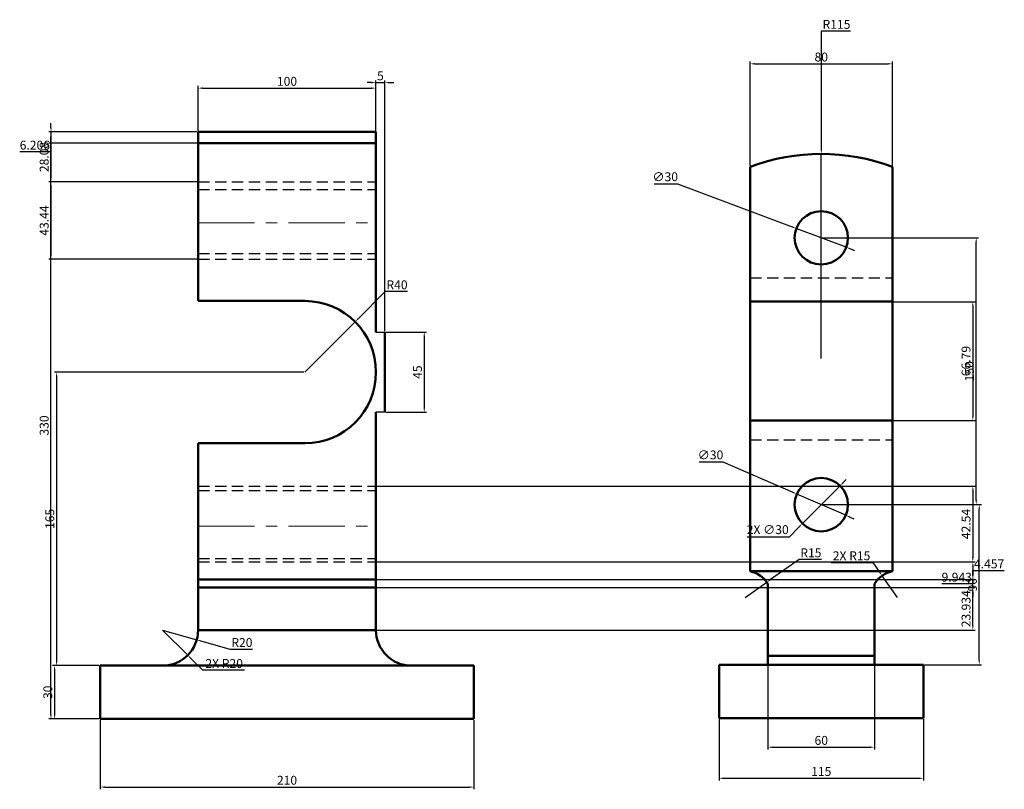
# Model space of a CAD drawing. Units: millimetres. Extents: x 1084 to 2343, y 1141 to 1965.
# Tile 2 of 4: x 1084 to 1638, y 1532 to 1965. Entities that reach past the tile are written whole.
import ezdxf

# ---------------------------------------------------------------- set-up
doc = ezdxf.new("R2010")
doc.units = ezdxf.units.MM
doc.linetypes.add('CENTER', pattern=[50.8, 31.75, -6.35, 6.35, -6.35])
doc.linetypes.add('HIDDEN', pattern=[9.525, 6.35, -3.175])
for name, color, linetype, lineweight in [('M-CNTR', 1, 'CENTER', 18), ('M-DIMS', 2, 'Continuous', 25), ('M-HIDN', 8, 'HIDDEN', 25), ('M-OUTL', 7, 'Continuous', 50)]:
    doc.layers.add(name, color=color, linetype=linetype, lineweight=lineweight)
doc.styles.get("Standard").update_dxf_attribs({"font": 'arial.ttf'})
doc.dimstyles.new('ISO-25', dxfattribs={"dimtxt": 5, "dimasz": 2.5, "dimexe": 1.25, "dimexo": 0.625, "dimtad": 1, "dimtoh": 1, "dimdec": 0, "dimtxsty": 'Standard', "dimcen": 2.5, "dimadec": 0, "dimazin": 0, "dimtfac": 1, "dimtdec": 0, "dimtmove": 0, "dimatfit": 3, "dimfxl": 1, "dimarcsym": 0})

# ---------------------------------------------------------------- blocks, each defined once
blk = doc.blocks.new('*D1')
at = {"layer": 'Defpoints', "color": 0, "transparency": 16777216}
for p in [(1129.73, 1571.53), (1339.73, 1571.53), (1339.73, 1533.25)]:
    blk.add_point(p, dxfattribs=at)
at = {"layer": 'M-DIMS', "color": 0, "lineweight": -2, "transparency": 16777216}
for p, q in [((1129.73, 1570.9), (1129.73, 1532)), ((1339.73, 1570.9), (1339.73, 1532)), ((1132.23, 1533.25), (1337.23, 1533.25))]:
    blk.add_line(p, q, dxfattribs=at)
at = {"layer": 'M-DIMS', "color": 0, "transparency": 16777216}
for points in [[(1132.23, 1533.67), (1132.23, 1532.84), (1129.73, 1533.25)], [(1337.23, 1533.67), (1337.23, 1532.84), (1339.73, 1533.25)]]:
    blk.add_solid(points, dxfattribs=at)
at = {"layer": 'M-DIMS', "color": 0, "transparency": 16777216, "insert": (1234.73, 1536.43), "char_height": 5, "attachment_point": 5}
blk.add_mtext('210', dxfattribs=at)
blk = doc.blocks.new('*D2')
at = {"layer": 'Defpoints', "color": 0, "transparency": 16777216}
for p in [(1129.73, 1601.53), (1104.02, 1571.53), (1129.73, 1571.53)]:
    blk.add_point(p, dxfattribs=at)
at = {"layer": 'M-DIMS', "color": 0, "lineweight": -2, "transparency": 16777216}
for p, q in [((1129.1, 1601.53), (1102.77, 1601.53)), ((1104.02, 1599.03), (1104.02, 1574.03)), ((1129.1, 1571.53), (1102.77, 1571.53))]:
    blk.add_line(p, q, dxfattribs=at)
at = {"layer": 'M-DIMS', "color": 0, "transparency": 16777216}
for points in [[(1103.6, 1599.03), (1104.44, 1599.03), (1104.02, 1601.53)], [(1103.6, 1574.03), (1104.44, 1574.03), (1104.02, 1571.53)]]:
    blk.add_solid(points, dxfattribs=at)
at = {"layer": 'M-DIMS', "color": 0, "transparency": 16777216, "insert": (1100.84, 1586.53), "char_height": 5, "attachment_point": 5, "rotation": 90}
blk.add_mtext('30', dxfattribs=at)
blk = doc.blocks.new('*D3')
at = {"layer": 'Defpoints', "color": 0, "transparency": 16777216}
for p in [(1244.73, 1766.53), (1105.16, 1601.53), (1129.73, 1601.53)]:
    blk.add_point(p, dxfattribs=at)
at = {"layer": 'M-DIMS', "color": 0, "lineweight": -2, "transparency": 16777216}
for p, q in [((1244.1, 1766.53), (1103.91, 1766.53)), ((1105.16, 1764.03), (1105.16, 1604.03)), ((1129.1, 1601.53), (1103.91, 1601.53))]:
    blk.add_line(p, q, dxfattribs=at)
at = {"layer": 'M-DIMS', "color": 0, "transparency": 16777216}
for points in [[(1104.74, 1764.03), (1105.57, 1764.03), (1105.16, 1766.53)], [(1104.74, 1604.03), (1105.57, 1604.03), (1105.16, 1601.53)]]:
    blk.add_solid(points, dxfattribs=at)
at = {"layer": 'M-DIMS', "color": 0, "transparency": 16777216, "insert": (1101.98, 1684.03), "char_height": 5, "attachment_point": 5, "rotation": 90}
blk.add_mtext('165', dxfattribs=at)
blk = doc.blocks.new('*D4')
at = {"layer": 'Defpoints', "color": 0, "transparency": 16777216}
for p in [(1289.73, 1789.03), (1289.73, 1744.03), (1311.91, 1744.03)]:
    blk.add_point(p, dxfattribs=at)
at = {"layer": 'M-DIMS', "color": 0, "lineweight": -2, "transparency": 16777216}
for p, q in [((1290.35, 1789.03), (1313.16, 1789.03)), ((1311.91, 1786.53), (1311.91, 1746.53)), ((1290.35, 1744.03), (1313.16, 1744.03))]:
    blk.add_line(p, q, dxfattribs=at)
at = {"layer": 'M-DIMS', "color": 0, "transparency": 16777216}
for points in [[(1311.49, 1786.53), (1312.32, 1786.53), (1311.91, 1789.03)], [(1311.49, 1746.53), (1312.32, 1746.53), (1311.91, 1744.03)]]:
    blk.add_solid(points, dxfattribs=at)
at = {"layer": 'M-DIMS', "color": 0, "transparency": 16777216, "insert": (1308.74, 1766.53), "char_height": 5, "attachment_point": 5, "rotation": 90}
blk.add_mtext('45', dxfattribs=at)
blk = doc.blocks.new('*D5')
at = {"layer": 'Defpoints', "color": 0, "transparency": 16777216}
for p in [(1284.73, 1926.18), (1184.73, 1901.53), (1284.73, 1901.53)]:
    blk.add_point(p, dxfattribs=at)
at = {"layer": 'M-DIMS', "color": 0, "lineweight": -2, "transparency": 16777216}
for p, q in [((1184.73, 1902.15), (1184.73, 1927.43)), ((1284.73, 1902.15), (1284.73, 1927.43)), ((1187.23, 1926.18), (1282.23, 1926.18))]:
    blk.add_line(p, q, dxfattribs=at)
at = {"layer": 'M-DIMS', "color": 0, "transparency": 16777216}
for points in [[(1187.23, 1926.6), (1187.23, 1925.76), (1184.73, 1926.18)], [(1282.23, 1926.6), (1282.23, 1925.76), (1284.73, 1926.18)]]:
    blk.add_solid(points, dxfattribs=at)
at = {"layer": 'M-DIMS', "color": 0, "transparency": 16777216, "insert": (1234.73, 1929.36), "char_height": 5, "attachment_point": 5}
blk.add_mtext('100', dxfattribs=at)
blk = doc.blocks.new('*D6')
at = {"layer": 'Defpoints', "color": 0, "transparency": 16777216}
for p in [(1164.73, 1621.53), (1183.96, 1616.04)]:
    blk.add_point(p, dxfattribs=at)
at = {"layer": 'M-DIMS', "color": 0, "lineweight": -2, "transparency": 16777216}
for p, q in [((1164.73, 1621.53), (1183.96, 1616.04)), ((1202.75, 1610.68), (1186.36, 1615.35)), ((1215.3, 1610.68), (1202.75, 1610.68))]:
    blk.add_line(p, q, dxfattribs=at)
at = {"layer": 'M-DIMS', "color": 0, "transparency": 16777216}
blk.add_solid([(1186.48, 1615.75), (1186.25, 1614.95), (1183.96, 1616.04)], dxfattribs=at)
at = {"layer": 'M-DIMS', "color": 0, "transparency": 16777216, "insert": (1209.34, 1613.86), "char_height": 5, "attachment_point": 5}
blk.add_mtext('R20', dxfattribs=at)
blk = doc.blocks.new('*D7')
at = {"layer": 'Defpoints', "color": 0, "transparency": 16777216}
for p in [(1477.66, 1572.02), (1592.66, 1572.02), (1592.66, 1538.19)]:
    blk.add_point(p, dxfattribs=at)
at = {"layer": 'M-DIMS', "color": 0, "lineweight": -2, "transparency": 16777216}
for p, q in [((1477.66, 1571.39), (1477.66, 1536.94)), ((1592.66, 1571.39), (1592.66, 1536.94)), ((1480.16, 1538.19), (1590.16, 1538.19))]:
    blk.add_line(p, q, dxfattribs=at)
at = {"layer": 'M-DIMS', "color": 0, "transparency": 16777216}
for points in [[(1480.16, 1538.6), (1480.16, 1537.77), (1477.66, 1538.19)], [(1590.16, 1538.6), (1590.16, 1537.77), (1592.66, 1538.19)]]:
    blk.add_solid(points, dxfattribs=at)
at = {"layer": 'M-DIMS', "color": 0, "transparency": 16777216, "insert": (1535.16, 1541.37), "char_height": 5, "attachment_point": 5}
blk.add_mtext('115', dxfattribs=at)
blk = doc.blocks.new('*D8')
at = {"layer": 'Defpoints', "color": 0, "transparency": 16777216}
for p in [(1505.16, 1602.02), (1565.16, 1602.02), (1565.16, 1555.67)]:
    blk.add_point(p, dxfattribs=at)
at = {"layer": 'M-DIMS', "color": 0, "lineweight": -2, "transparency": 16777216}
for p, q in [((1505.16, 1601.39), (1505.16, 1554.42)), ((1565.16, 1601.39), (1565.16, 1554.42)), ((1507.66, 1555.67), (1562.66, 1555.67))]:
    blk.add_line(p, q, dxfattribs=at)
at = {"layer": 'M-DIMS', "color": 0, "transparency": 16777216}
for points in [[(1507.66, 1556.09), (1507.66, 1555.25), (1505.16, 1555.67)], [(1562.66, 1556.09), (1562.66, 1555.25), (1565.16, 1555.67)]]:
    blk.add_solid(points, dxfattribs=at)
at = {"layer": 'M-DIMS', "color": 0, "transparency": 16777216, "insert": (1535.16, 1558.85), "char_height": 5, "attachment_point": 5}
blk.add_mtext('60', dxfattribs=at)
blk = doc.blocks.new('*D9')
at = {"layer": 'Defpoints', "color": 0, "transparency": 16777216}
for p in [(1535.16, 1692.02), (1624, 1692.02), (1592.66, 1602.02)]:
    blk.add_point(p, dxfattribs=at)
at = {"layer": 'M-DIMS', "color": 0, "lineweight": -2, "transparency": 16777216}
for p, q in [((1535.78, 1692.02), (1625.25, 1692.02)), ((1624, 1604.52), (1624, 1689.52)), ((1593.28, 1602.02), (1625.25, 1602.02))]:
    blk.add_line(p, q, dxfattribs=at)
at = {"layer": 'M-DIMS', "color": 0, "transparency": 16777216}
for points in [[(1623.58, 1689.52), (1624.42, 1689.52), (1624, 1692.02)], [(1623.58, 1604.52), (1624.42, 1604.52), (1624, 1602.02)]]:
    blk.add_solid(points, dxfattribs=at)
at = {"layer": 'M-DIMS', "color": 0, "transparency": 16777216, "insert": (1620.82, 1647.02), "char_height": 5, "attachment_point": 5, "rotation": 90}
blk.add_mtext('90', dxfattribs=at)
blk = doc.blocks.new('*D10')
at = {"layer": 'Defpoints', "color": 0, "transparency": 16777216}
for p in [(1535.16, 1842.02), (1622.3, 1842.02), (1535.16, 1692.02)]:
    blk.add_point(p, dxfattribs=at)
at = {"layer": 'M-DIMS', "color": 0, "lineweight": -2, "transparency": 16777216}
for p, q in [((1535.78, 1842.02), (1623.55, 1842.02)), ((1622.3, 1694.52), (1622.3, 1839.52)), ((1535.78, 1692.02), (1623.55, 1692.02))]:
    blk.add_line(p, q, dxfattribs=at)
at = {"layer": 'M-DIMS', "color": 0, "transparency": 16777216}
for points in [[(1621.89, 1839.52), (1622.72, 1839.52), (1622.3, 1842.02)], [(1621.89, 1694.52), (1622.72, 1694.52), (1622.3, 1692.02)]]:
    blk.add_solid(points, dxfattribs=at)
at = {"layer": 'M-DIMS', "color": 0, "transparency": 16777216, "insert": (1619.12, 1767.02), "char_height": 5, "attachment_point": 5, "rotation": 90}
blk.add_mtext('150', dxfattribs=at)
blk = doc.blocks.new('*D11')
at = {"layer": 'Defpoints', "color": 0, "transparency": 16777216}
for p in [(1575.16, 1939.86), (1495.16, 1882.02), (1575.16, 1882.02)]:
    blk.add_point(p, dxfattribs=at)
at = {"layer": 'M-DIMS', "color": 0, "lineweight": -2, "transparency": 16777216}
for p, q in [((1495.16, 1882.64), (1495.16, 1941.11)), ((1497.66, 1939.86), (1572.66, 1939.86)), ((1575.16, 1882.64), (1575.16, 1941.11))]:
    blk.add_line(p, q, dxfattribs=at)
at = {"layer": 'M-DIMS', "color": 0, "transparency": 16777216}
for points in [[(1497.66, 1940.27), (1497.66, 1939.44), (1495.16, 1939.86)], [(1572.66, 1940.27), (1572.66, 1939.44), (1575.16, 1939.86)]]:
    blk.add_solid(points, dxfattribs=at)
at = {"layer": 'M-DIMS', "color": 0, "transparency": 16777216, "insert": (1535.16, 1943.03), "char_height": 5, "attachment_point": 5}
blk.add_mtext('80', dxfattribs=at)
blk = doc.blocks.new('*D12')
at = {"layer": 'Defpoints', "color": 0, "transparency": 16777216}
for p in [(1521.12, 1847.3), (1549.2, 1836.74)]:
    blk.add_point(p, dxfattribs=at)
at = {"layer": 'M-DIMS', "color": 0, "lineweight": -2, "transparency": 16777216}
for p, q in [((1441.13, 1872.4), (1454.34, 1872.4)), ((1454.34, 1872.4), (1518.78, 1848.18)), ((1549.2, 1836.74), (1521.12, 1847.3)), ((1551.54, 1835.86), (1553.88, 1834.98))]:
    blk.add_line(p, q, dxfattribs=at)
at = {"layer": 'M-DIMS', "color": 0, "transparency": 16777216}
for points in [[(1518.93, 1848.57), (1518.63, 1847.79), (1521.12, 1847.3)], [(1551.69, 1836.25), (1551.39, 1835.47), (1549.2, 1836.74)]]:
    blk.add_solid(points, dxfattribs=at)
at = {"layer": 'M-DIMS', "color": 0, "transparency": 16777216, "insert": (1447.42, 1875.72), "char_height": 5, "attachment_point": 5}
blk.add_mtext('∅30', dxfattribs=at)
blk = doc.blocks.new('*D13')
at = {"layer": 'Defpoints', "color": 0, "transparency": 16777216}
for p in [(1521.4, 1697.99), (1548.92, 1686.05)]:
    blk.add_point(p, dxfattribs=at)
at = {"layer": 'M-DIMS', "color": 0, "lineweight": -2, "transparency": 16777216}
for p, q in [((1466.57, 1716.04), (1479.78, 1716.04)), ((1479.78, 1716.04), (1519.1, 1698.98)), ((1548.92, 1686.05), (1521.4, 1697.99)), ((1551.21, 1685.06), (1553.51, 1684.06))]:
    blk.add_line(p, q, dxfattribs=at)
at = {"layer": 'M-DIMS', "color": 0, "transparency": 16777216}
for points in [[(1519.27, 1699.37), (1518.94, 1698.6), (1521.4, 1697.99)], [(1551.38, 1685.44), (1551.05, 1684.67), (1548.92, 1686.05)]]:
    blk.add_solid(points, dxfattribs=at)
at = {"layer": 'M-DIMS', "color": 0, "transparency": 16777216, "insert": (1472.87, 1719.35), "char_height": 5, "attachment_point": 5}
blk.add_mtext('∅30', dxfattribs=at)
blk = doc.blocks.new('*D14')
at = {"layer": 'Defpoints', "color": 0, "transparency": 16777216}
for p in [(1504.58, 1648.42), (1492.29, 1639.82)]:
    blk.add_point(p, dxfattribs=at)
at = {"layer": 'M-DIMS', "color": 0, "lineweight": -2, "transparency": 16777216}
for p, q in [((1522.72, 1661.12), (1506.63, 1649.86)), ((1535.33, 1661.12), (1522.72, 1661.12)), ((1492.29, 1639.82), (1504.58, 1648.42))]:
    blk.add_line(p, q, dxfattribs=at)
at = {"layer": 'M-DIMS', "color": 0, "transparency": 16777216}
blk.add_solid([(1506.39, 1650.2), (1506.87, 1649.51), (1504.58, 1648.42)], dxfattribs=at)
at = {"layer": 'M-DIMS', "color": 0, "transparency": 16777216, "insert": (1529.34, 1664.3), "char_height": 5, "attachment_point": 5}
blk.add_mtext('R15', dxfattribs=at)
blk = doc.blocks.new('*D48')
at = {"layer": 'Defpoints', "color": 0, "transparency": 16777216}
for p in [(1101.98, 1901.53), (1184.73, 1901.53), (1129.73, 1571.53)]:
    blk.add_point(p, dxfattribs=at)
at = {"layer": 'M-DIMS', "color": 0, "lineweight": -2, "transparency": 16777216}
for p, q in [((1184.1, 1901.53), (1100.73, 1901.53)), ((1101.98, 1574.03), (1101.98, 1899.03)), ((1129.1, 1571.53), (1100.73, 1571.53))]:
    blk.add_line(p, q, dxfattribs=at)
at = {"layer": 'M-DIMS', "color": 0, "transparency": 16777216}
for points in [[(1101.56, 1899.03), (1102.39, 1899.03), (1101.98, 1901.53)], [(1101.56, 1574.03), (1102.39, 1574.03), (1101.98, 1571.53)]]:
    blk.add_solid(points, dxfattribs=at)
at = {"layer": 'M-DIMS', "color": 0, "transparency": 16777216, "insert": (1098.8, 1736.53), "char_height": 5, "attachment_point": 5, "rotation": 90}
blk.add_mtext('330', dxfattribs=at)
blk = doc.blocks.new('*D49')
at = {"layer": 'Defpoints', "color": 0, "transparency": 16777216}
for p in [(1184.73, 1901.53), (1101.98, 1895.32), (1184.73, 1895.32)]:
    blk.add_point(p, dxfattribs=at)
at = {"layer": 'M-DIMS', "color": 0, "lineweight": -2, "transparency": 16777216}
for p, q in [((1101.98, 1904.03), (1101.98, 1906.53)), ((1184.1, 1901.53), (1100.73, 1901.53)), ((1101.98, 1901.53), (1101.98, 1895.32)), ((1184.1, 1895.32), (1100.73, 1895.32)), ((1101.98, 1890.32), (1084.46, 1890.32)), ((1101.98, 1892.82), (1101.98, 1890.32))]:
    blk.add_line(p, q, dxfattribs=at)
at = {"layer": 'M-DIMS', "color": 0, "transparency": 16777216}
for points in [[(1101.56, 1904.03), (1102.39, 1904.03), (1101.98, 1901.53)], [(1101.56, 1892.82), (1102.39, 1892.82), (1101.98, 1895.32)]]:
    blk.add_solid(points, dxfattribs=at)
at = {"layer": 'M-DIMS', "color": 0, "transparency": 16777216, "insert": (1092.9, 1893.5), "char_height": 5, "attachment_point": 5}
blk.add_mtext('6.206', dxfattribs=at)
blk = doc.blocks.new('*D50')
at = {"layer": 'Defpoints', "color": 0, "transparency": 16777216}
for p in [(1289.73, 1929.28), (1284.73, 1789.03), (1289.73, 1789.03)]:
    blk.add_point(p, dxfattribs=at)
at = {"layer": 'M-DIMS', "color": 0, "lineweight": -2, "transparency": 16777216}
for p, q in [((1282.23, 1929.28), (1279.73, 1929.28)), ((1284.73, 1789.65), (1284.73, 1930.53)), ((1284.73, 1929.28), (1289.73, 1929.28)), ((1289.73, 1789.65), (1289.73, 1930.53)), ((1292.23, 1929.28), (1294.73, 1929.28))]:
    blk.add_line(p, q, dxfattribs=at)
at = {"layer": 'M-DIMS', "color": 0, "transparency": 16777216}
for points in [[(1282.23, 1929.69), (1282.23, 1928.86), (1284.73, 1929.28)], [(1292.23, 1929.69), (1292.23, 1928.86), (1289.73, 1929.28)]]:
    blk.add_solid(points, dxfattribs=at)
at = {"layer": 'M-DIMS', "color": 0, "transparency": 16777216, "insert": (1287.23, 1932.45), "char_height": 5, "attachment_point": 5}
blk.add_mtext('5', dxfattribs=at)
blk = doc.blocks.new('*D51')
at = {"layer": 'Defpoints', "color": 0, "transparency": 16777216}
for p in [(1284.73, 1645.46), (1620.41, 1645.46), (1284.73, 1621.53)]:
    blk.add_point(p, dxfattribs=at)
at = {"layer": 'M-DIMS', "color": 0, "lineweight": -2, "transparency": 16777216}
for p, q in [((1285.35, 1645.46), (1621.66, 1645.46)), ((1620.41, 1624.03), (1620.41, 1642.96)), ((1285.35, 1621.53), (1621.66, 1621.53))]:
    blk.add_line(p, q, dxfattribs=at)
at = {"layer": 'M-DIMS', "color": 0, "transparency": 16777216}
for points in [[(1619.99, 1642.96), (1620.83, 1642.96), (1620.41, 1645.46)], [(1619.99, 1624.03), (1620.83, 1624.03), (1620.41, 1621.53)]]:
    blk.add_solid(points, dxfattribs=at)
at = {"layer": 'M-DIMS', "color": 0, "transparency": 16777216, "insert": (1617.23, 1633.5), "char_height": 5, "attachment_point": 5, "rotation": 90}
blk.add_mtext('23.934', dxfattribs=at)
blk = doc.blocks.new('*D52')
at = {"layer": 'Defpoints', "color": 0, "transparency": 16777216}
for p in [(1284.73, 1649.92), (1284.73, 1645.46), (1620.41, 1649.92)]:
    blk.add_point(p, dxfattribs=at)
at = {"layer": 'M-DIMS', "color": 0, "lineweight": -2, "transparency": 16777216}
for p, q in [((1620.41, 1652.42), (1620.41, 1654.92)), ((1620.41, 1654.92), (1638.11, 1654.92)), ((1285.35, 1649.92), (1621.66, 1649.92)), ((1285.35, 1645.46), (1621.66, 1645.46)), ((1620.41, 1645.46), (1620.41, 1649.92)), ((1620.41, 1642.96), (1620.41, 1640.46))]:
    blk.add_line(p, q, dxfattribs=at)
at = {"layer": 'M-DIMS', "color": 0, "transparency": 16777216}
for points in [[(1619.99, 1652.42), (1620.83, 1652.42), (1620.41, 1649.92)], [(1619.99, 1642.96), (1620.83, 1642.96), (1620.41, 1645.46)]]:
    blk.add_solid(points, dxfattribs=at)
at = {"layer": 'M-DIMS', "color": 0, "transparency": 16777216, "insert": (1629.57, 1658.09), "char_height": 5, "attachment_point": 5}
blk.add_mtext('4.457', dxfattribs=at)
blk = doc.blocks.new('*D53')
at = {"layer": 'Defpoints', "color": 0, "transparency": 16777216}
for p in [(1184.73, 1901.53), (1101.98, 1873.45), (1184.73, 1873.45)]:
    blk.add_point(p, dxfattribs=at)
at = {"layer": 'M-DIMS', "color": 0, "lineweight": -2, "transparency": 16777216}
for p, q in [((1184.1, 1901.53), (1100.73, 1901.53)), ((1101.98, 1899.03), (1101.98, 1875.95)), ((1184.1, 1873.45), (1100.73, 1873.45))]:
    blk.add_line(p, q, dxfattribs=at)
at = {"layer": 'M-DIMS', "color": 0, "transparency": 16777216}
for points in [[(1101.56, 1899.03), (1102.39, 1899.03), (1101.98, 1901.53)], [(1101.56, 1875.95), (1102.39, 1875.95), (1101.98, 1873.45)]]:
    blk.add_solid(points, dxfattribs=at)
at = {"layer": 'M-DIMS', "color": 0, "transparency": 16777216, "insert": (1098.8, 1887.49), "char_height": 5, "attachment_point": 5, "rotation": 90}
blk.add_mtext('28.08', dxfattribs=at)
blk = doc.blocks.new('*D54')
at = {"layer": 'Defpoints', "color": 0, "transparency": 16777216}
for p in [(1184.73, 1873.45), (1101.98, 1830.01), (1184.73, 1830.01)]:
    blk.add_point(p, dxfattribs=at)
at = {"layer": 'M-DIMS', "color": 0, "lineweight": -2, "transparency": 16777216}
for p, q in [((1184.1, 1873.45), (1100.73, 1873.45)), ((1101.98, 1870.95), (1101.98, 1832.51)), ((1184.1, 1830.01), (1100.73, 1830.01))]:
    blk.add_line(p, q, dxfattribs=at)
at = {"layer": 'M-DIMS', "color": 0, "transparency": 16777216}
for points in [[(1101.56, 1870.95), (1102.39, 1870.95), (1101.98, 1873.45)], [(1101.56, 1832.51), (1102.39, 1832.51), (1101.98, 1830.01)]]:
    blk.add_solid(points, dxfattribs=at)
at = {"layer": 'M-DIMS', "color": 0, "transparency": 16777216, "insert": (1098.8, 1851.73), "char_height": 5, "attachment_point": 5, "rotation": 90}
blk.add_mtext('43.44', dxfattribs=at)
blk = doc.blocks.new('*D55')
at = {"layer": 'Defpoints', "color": 0, "transparency": 16777216}
for p in [(1284.73, 1702.41), (1284.73, 1659.86), (1620.41, 1659.86)]:
    blk.add_point(p, dxfattribs=at)
at = {"layer": 'M-DIMS', "color": 0, "lineweight": -2, "transparency": 16777216}
for p, q in [((1285.35, 1702.41), (1621.66, 1702.41)), ((1620.41, 1699.91), (1620.41, 1662.36)), ((1285.35, 1659.86), (1621.66, 1659.86))]:
    blk.add_line(p, q, dxfattribs=at)
at = {"layer": 'M-DIMS', "color": 0, "transparency": 16777216}
for points in [[(1619.99, 1699.91), (1620.83, 1699.91), (1620.41, 1702.41)], [(1619.99, 1662.36), (1620.83, 1662.36), (1620.41, 1659.86)]]:
    blk.add_solid(points, dxfattribs=at)
at = {"layer": 'M-DIMS', "color": 0, "transparency": 16777216, "insert": (1617.23, 1681.13), "char_height": 5, "attachment_point": 5, "rotation": 90}
blk.add_mtext('42.54', dxfattribs=at)
blk = doc.blocks.new('*D56')
at = {"layer": 'Defpoints', "color": 0, "transparency": 16777216}
for p in [(1284.73, 1659.86), (1284.73, 1649.92), (1620.41, 1649.92)]:
    blk.add_point(p, dxfattribs=at)
at = {"layer": 'M-DIMS', "color": 0, "lineweight": -2, "transparency": 16777216}
for p, q in [((1285.35, 1659.86), (1621.66, 1659.86)), ((1620.41, 1657.36), (1620.41, 1652.42)), ((1285.35, 1649.92), (1621.66, 1649.92)), ((1620.41, 1647.42), (1602.91, 1647.42)), ((1620.41, 1649.92), (1620.41, 1647.42))]:
    blk.add_line(p, q, dxfattribs=at)
at = {"layer": 'M-DIMS', "color": 0, "transparency": 16777216}
for points in [[(1619.99, 1657.36), (1620.83, 1657.36), (1620.41, 1659.86)], [(1619.99, 1652.42), (1620.83, 1652.42), (1620.41, 1649.92)]]:
    blk.add_solid(points, dxfattribs=at)
at = {"layer": 'M-DIMS', "color": 0, "transparency": 16777216, "insert": (1611.35, 1650.6), "char_height": 5, "attachment_point": 5}
blk.add_mtext('9.943', dxfattribs=at)
blk = doc.blocks.new('*D57')
at = {"layer": 'Defpoints', "color": 0, "transparency": 16777216}
for p in [(1575.16, 1806.14), (1575.16, 1739.35), (1620.41, 1739.35)]:
    blk.add_point(p, dxfattribs=at)
at = {"layer": 'M-DIMS', "color": 0, "lineweight": -2, "transparency": 16777216}
for p, q in [((1575.78, 1806.14), (1621.66, 1806.14)), ((1620.41, 1803.64), (1620.41, 1741.85)), ((1575.78, 1739.35), (1621.66, 1739.35))]:
    blk.add_line(p, q, dxfattribs=at)
at = {"layer": 'M-DIMS', "color": 0, "transparency": 16777216}
for points in [[(1619.99, 1803.64), (1620.83, 1803.64), (1620.41, 1806.14)], [(1619.99, 1741.85), (1620.83, 1741.85), (1620.41, 1739.35)]]:
    blk.add_solid(points, dxfattribs=at)
at = {"layer": 'M-DIMS', "color": 0, "transparency": 16777216, "insert": (1617.23, 1772.75), "char_height": 5, "attachment_point": 5, "rotation": 90}
blk.add_mtext('66.79', dxfattribs=at)
blk = doc.blocks.new('*D69')
at = {"layer": 'Defpoints', "color": 0, "transparency": 16777216}
for p in [(1273.01, 1794.81), (1244.73, 1766.53)]:
    blk.add_point(p, dxfattribs=at)
at = {"layer": 'M-DIMS', "color": 0, "lineweight": -2, "transparency": 16777216}
for p, q in [((1289.98, 1811.78), (1274.78, 1796.58)), ((1302.54, 1811.78), (1289.98, 1811.78)), ((1244.73, 1766.53), (1273.01, 1794.81))]:
    blk.add_line(p, q, dxfattribs=at)
at = {"layer": 'M-DIMS', "color": 0, "transparency": 16777216}
blk.add_solid([(1274.48, 1796.87), (1275.07, 1796.28), (1273.01, 1794.81)], dxfattribs=at)
at = {"layer": 'M-DIMS', "color": 0, "transparency": 16777216, "insert": (1296.57, 1814.96), "char_height": 5, "attachment_point": 5}
blk.add_mtext('R40', dxfattribs=at)
blk = doc.blocks.new('*D70')
at = {"layer": 'Defpoints', "color": 0, "transparency": 16777216}
for p in [(1164.73, 1621.53), (1178.87, 1607.39)]:
    blk.add_point(p, dxfattribs=at)
at = {"layer": 'M-DIMS', "color": 0, "lineweight": -2, "transparency": 16777216}
for p, q in [((1164.73, 1621.53), (1178.87, 1607.39)), ((1187.36, 1598.9), (1180.64, 1605.62)), ((1210.74, 1598.9), (1187.36, 1598.9))]:
    blk.add_line(p, q, dxfattribs=at)
at = {"layer": 'M-DIMS', "color": 0, "transparency": 16777216}
blk.add_solid([(1180.93, 1605.92), (1180.34, 1605.33), (1178.87, 1607.39)], dxfattribs=at)
at = {"layer": 'M-DIMS', "color": 0, "transparency": 16777216, "insert": (1199.36, 1602.08), "char_height": 5, "attachment_point": 5}
blk.add_mtext('2X R20', dxfattribs=at)
blk = doc.blocks.new('*D71')
at = {"layer": 'Defpoints', "color": 0, "transparency": 16777216}
for p in [(1535.16, 1889.2), (1535.16, 1774.2)]:
    blk.add_point(p, dxfattribs=at)
at = {"layer": 'M-DIMS', "color": 0, "lineweight": -2, "transparency": 16777216}
for p, q in [((1551.66, 1958.2), (1535.16, 1958.2)), ((1535.16, 1958.2), (1535.16, 1891.7)), ((1535.16, 1774.2), (1535.16, 1889.2))]:
    blk.add_line(p, q, dxfattribs=at)
at = {"layer": 'M-DIMS', "color": 0, "transparency": 16777216}
blk.add_solid([(1534.74, 1891.7), (1535.58, 1891.7), (1535.16, 1889.2)], dxfattribs=at)
at = {"layer": 'M-DIMS', "color": 0, "transparency": 16777216, "insert": (1543.72, 1961.38), "char_height": 5, "attachment_point": 5}
blk.add_mtext('R115', dxfattribs=at)
blk = doc.blocks.new('*D72')
at = {"layer": 'Defpoints', "color": 0, "transparency": 16777216}
for p in [(1545.74, 1702.66), (1524.58, 1681.38)]:
    blk.add_point(p, dxfattribs=at)
at = {"layer": 'M-DIMS', "color": 0, "lineweight": -2, "transparency": 16777216}
for p, q in [((1547.5, 1704.43), (1549.26, 1706.2)), ((1545.74, 1702.66), (1524.58, 1681.38)), ((1517.26, 1674.02), (1522.82, 1679.61)), ((1493.49, 1674.02), (1517.26, 1674.02))]:
    blk.add_line(p, q, dxfattribs=at)
at = {"layer": 'M-DIMS', "color": 0, "transparency": 16777216}
for points in [[(1547.2, 1704.72), (1547.79, 1704.14), (1545.74, 1702.66)], [(1522.52, 1679.9), (1523.12, 1679.32), (1524.58, 1681.38)]]:
    blk.add_solid(points, dxfattribs=at)
at = {"layer": 'M-DIMS', "color": 0, "transparency": 16777216, "insert": (1505.06, 1677.34), "char_height": 5, "attachment_point": 5}
blk.add_mtext('2X ∅30', dxfattribs=at)
blk = doc.blocks.new('*D73')
at = {"layer": 'Defpoints', "color": 0, "transparency": 16777216}
for p in [(1569.41, 1652.1), (1578.03, 1639.82)]:
    blk.add_point(p, dxfattribs=at)
at = {"layer": 'M-DIMS', "color": 0, "lineweight": -2, "transparency": 16777216}
for p, q in [((1540.8, 1659.47), (1564.24, 1659.47)), ((1564.24, 1659.47), (1567.97, 1654.15)), ((1578.03, 1639.82), (1569.41, 1652.1))]:
    blk.add_line(p, q, dxfattribs=at)
at = {"layer": 'M-DIMS', "color": 0, "transparency": 16777216}
blk.add_solid([(1568.32, 1654.38), (1567.63, 1653.91), (1569.41, 1652.1)], dxfattribs=at)
at = {"layer": 'M-DIMS', "color": 0, "transparency": 16777216, "insert": (1552.21, 1662.64), "char_height": 5, "attachment_point": 5}
blk.add_mtext('2X R15', dxfattribs=at)

msp = doc.modelspace()

# ---------------------------------------------------------------- linework, layer by layer
at = {"layer": 'M-CNTR'}
for p, q in [((1184.7265, 1850.3705), (1284.7265, 1850.3705)), ((1184.7265, 1679.9449), (1284.7265, 1679.9449))]:
    msp.add_line(p, q, dxfattribs=at)
at = {"layer": 'M-HIDN'}
for p, q in [((1184.7265, 1873.4476), (1284.7265, 1873.4476)), ((1184.7265, 1869.2313), (1284.7265, 1869.2313)), ((1184.7265, 1833.2243), (1284.7265, 1833.2243)), ((1184.7265, 1830.0094), (1284.7265, 1830.0094)), ((1495.1592, 1819.4554), (1575.1592, 1819.4554)), ((1284.7265, 1789.028), (1289.7265, 1789.028)), ((1289.7265, 1744.028), (1284.7265, 1744.028)), ((1495.1592, 1728.4089), (1575.1592, 1728.4089)), ((1184.7265, 1702.4059), (1284.7265, 1702.4059)), ((1184.7265, 1699.9672), (1284.7265, 1699.9672)), ((1184.7265, 1661.7357), (1284.7265, 1661.7357)), ((1184.7265, 1659.8623), (1284.7265, 1659.8623))]:
    msp.add_line(p, q, dxfattribs=at)
at = {"layer": 'M-OUTL'}
for p, q in [((1184.7265, 1901.528), (1284.7265, 1901.528)), ((1184.7265, 1901.528), (1184.7265, 1806.528)), ((1284.7265, 1901.528), (1284.7265, 1789.028)), ((1184.7265, 1895.3218), (1284.7265, 1895.3218)), ((1495.1592, 1842.0194), (1495.1592, 1882.0194)), ((1575.1592, 1842.0194), (1575.1592, 1882.0194)), ((1495.1592, 1842.0194), (1495.1592, 1692.0194)), ((1575.1592, 1842.0194), (1575.1592, 1692.0194)), ((1186.4973, 1806.528), (1184.7265, 1806.528)), ((1244.7265, 1806.528), (1186.4973, 1806.528)), ((1495.1592, 1806.1449), (1575.1592, 1806.1449)), ((1289.7265, 1789.028), (1289.7265, 1744.028)), ((1284.7265, 1744.028), (1284.7265, 1621.528)), ((1495.1592, 1739.3534), (1575.1592, 1739.3534)), ((1184.7265, 1621.528), (1184.7265, 1726.528)), ((1244.7265, 1726.528), (1184.7265, 1726.528)), ((1495.1592, 1692.0194), (1495.1592, 1654.5444)), ((1575.1592, 1692.0194), (1575.1592, 1654.5444)), ((1575.1592, 1654.5444), (1495.1592, 1654.5444)), ((1184.7265, 1649.9195), (1284.7265, 1649.9195)), ((1184.7265, 1645.4624), (1284.7265, 1645.4624)), ((1505.1592, 1602.0194), (1505.1592, 1647.5282)), ((1565.1592, 1602.0194), (1565.1592, 1647.5282)), ((1184.7265, 1621.528), (1284.7265, 1621.528)), ((1505.1592, 1602.0194), (1505.1592, 1607.0194)), ((1505.1592, 1607.0194), (1565.1592, 1607.0194)), ((1164.7265, 1601.528), (1129.7265, 1601.528)), ((1129.7265, 1601.528), (1129.7265, 1571.528)), ((1164.7265, 1601.528), (1304.7265, 1601.528)), ((1234.7265, 1601.528), (1184.7265, 1601.528)), ((1234.7265, 1601.528), (1234.7265, 1601.528)), ((1304.7265, 1601.528), (1339.7265, 1601.528)), ((1339.7265, 1571.528), (1339.7265, 1601.528)), ((1477.6592, 1602.0194), (1592.6592, 1602.0194)), ((1477.6592, 1572.0194), (1477.6592, 1602.0194)), ((1535.1592, 1602.0194), (1505.1592, 1602.0194)), ((1535.1592, 1602.0194), (1505.1592, 1602.0194)), ((1535.1592, 1602.0194), (1565.1592, 1602.0194)), ((1592.6592, 1602.0194), (1592.6592, 1572.0194)), ((1129.7265, 1571.528), (1339.7265, 1571.528)), ((1592.6592, 1572.0194), (1477.6592, 1572.0194))]:
    msp.add_line(p, q, dxfattribs=at)
for centre in [(1535.1592, 1842.0194), (1535.1592, 1692.0194)]:
    msp.add_circle(centre, 15, dxfattribs=at)
for centre, radius, start, end in [((1535.1592, 1774.2001), 115, 69.645594, 110.354406), ((1244.7265, 1766.528), 40, 270, 90), ((1492.2905, 1639.8212), 15, 30.917056, 78.974531), ((1578.0279, 1639.8212), 15, 101.025469, 149.082944), ((1164.7265, 1621.528), 20, 270, 0), ((1304.7265, 1621.528), 20, 180, 270)]:
    msp.add_arc(centre, radius, start, end, dxfattribs=at)

# ---------------------------------------------------------------- dimensions: what is measured, and where the dimension line sits
at = {"layer": 'M-DIMS'}
for center, mpoint, override, picture, middle in [((1535.1592, 1774.2001), (1535.16, 1889.2001), {"dimdec": 0, "dimlfac": 1, "dimrnd": 0, "dimzin": 0, "dimdsep": 46, "dimlunit": 2}, '*D71', (1543.7203, 1958.2001)), ((1244.7265, 1766.528), (1273.0115, 1794.8115), {"dimdec": 0, "dimlfac": 1, "dimrnd": 0, "dimzin": 0, "dimdsep": 46, "dimlunit": 2}, '*D69', (1296.5728, 1811.7816)), ((1492.2905, 1639.8212), (1504.5801, 1648.4217), {"dimclrd": 0, "dimclre": 0, "dimclrt": 0}, '*D14', (1529.3402, 1661.1181)), ((1164.7265, 1621.528), (1183.9587, 1616.0397), {"dimclrd": 0, "dimclre": 0, "dimclrt": 0}, '*D6', (1209.336, 1610.6784))]:
    dim = msp.add_radius_dim(center=center, mpoint=mpoint, dimstyle='ISO-25', override=override, dxfattribs=at)
    dim.commit()
    dim.dimension.update_dxf_attribs({"geometry": picture, "text_midpoint": middle, "dimtype": 164})
for base, p1, p2, override, picture, middle in [((1575.1592, 1939.8552), (1495.1592, 1882.0194), (1575.1592, 1882.0194), {"dimclrd": 0, "dimclre": 0, "dimclrt": 0}, '*D11', (1535.1592, 1943.0331)), ((1284.7265, 1926.1793), (1184.7265, 1901.528), (1284.7265, 1901.528), {"dimclrd": 0, "dimclre": 0, "dimclrt": 0}, '*D5', (1234.7265, 1929.3571)), ((1289.7265, 1929.278), (1284.7265, 1789.028), (1289.7265, 1789.028), {"dimdec": 0, "dimlfac": 1, "dimrnd": 0, "dimzin": 0, "dimdsep": 46, "dimlunit": 2}, '*D50', (1287.2265, 1932.4457)), ((1565.1592, 1555.671), (1505.1592, 1602.0194), (1565.1592, 1602.0194), {"dimclrd": 0, "dimclre": 0, "dimclrt": 0}, '*D8', (1535.1592, 1558.8489)), ((1339.7265, 1533.2531), (1129.7265, 1571.528), (1339.7265, 1571.528), {"dimclrd": 0, "dimclre": 0, "dimclrt": 0}, '*D1', (1234.7265, 1536.4309)), ((1592.6592, 1538.1882), (1477.6592, 1572.0194), (1592.6592, 1572.0194), {"dimclrd": 0, "dimclre": 0, "dimclrt": 0}, '*D7', (1535.1592, 1541.3661))]:
    dim = msp.add_linear_dim(base=base, p1=p1, p2=p2, dimstyle='ISO-25', override=override, dxfattribs=at)
    dim.commit()
    dim.dimension.update_dxf_attribs({"geometry": picture, "text_midpoint": middle})
for base, p1, p2, override, picture, middle in [((1101.9765, 1895.3218), (1184.7265, 1901.528), (1184.7265, 1895.3218), {"dimdec": 3, "dimlfac": 1, "dimrnd": 0, "dimzin": 0, "dimdsep": 46, "dimlunit": 2}, '*D49', (1092.9033, 1893.4996)), ((1101.9765, 1901.528), (1129.7265, 1571.528), (1184.7265, 1901.528), {"dimdec": 0, "dimlfac": 1, "dimrnd": 0, "dimzin": 0, "dimdsep": 46, "dimlunit": 2}, '*D48', (1098.7969, 1736.528)), ((1101.9765, 1873.4476), (1184.7265, 1901.528), (1184.7265, 1873.4476), {"dimdec": 2, "dimlfac": 1, "dimrnd": 0, "dimzin": 0, "dimdsep": 46, "dimlunit": 2}, '*D53', (1098.7986, 1887.4878)), ((1101.9765, 1830.0094), (1184.7265, 1873.4476), (1184.7265, 1830.0094), {"dimdec": 2, "dimlfac": 1, "dimrnd": 0, "dimzin": 0, "dimdsep": 46, "dimlunit": 2}, '*D54', (1098.7969, 1851.7285)), ((1622.3025, 1842.0194), (1535.1592, 1692.0194), (1535.1592, 1842.0194), {"dimclrd": 0, "dimclre": 0, "dimclrt": 0}, '*D10', (1619.1247, 1767.0194)), ((1620.4092, 1739.3534), (1575.1592, 1806.1449), (1575.1592, 1739.3534), {"dimdec": 2, "dimlfac": 1, "dimrnd": 0, "dimzin": 0, "dimdsep": 46, "dimlunit": 2}, '*D57', (1617.2314, 1772.7491)), ((1311.9073, 1744.028), (1289.7265, 1789.028), (1289.7265, 1744.028), {"dimclrd": 0, "dimclre": 0, "dimclrt": 0}, '*D4', (1308.7397, 1766.528)), ((1105.1578, 1601.528), (1244.7265, 1766.528), (1129.7265, 1601.528), {"dimclrd": 0, "dimclre": 0, "dimclrt": 0}, '*D3', (1101.9799, 1684.028)), ((1620.4092, 1659.8623), (1284.7265, 1702.4059), (1284.7265, 1659.8623), {"dimdec": 2, "dimlfac": 1, "dimrnd": 0, "dimzin": 0, "dimdsep": 46, "dimlunit": 2}, '*D55', (1617.2314, 1681.1341)), ((1624.0008, 1692.0194), (1592.6592, 1602.0194), (1535.1592, 1692.0194), {"dimclrd": 0, "dimclre": 0, "dimclrt": 0}, '*D9', (1620.823, 1647.0194)), ((1620.4092, 1649.9195), (1284.7265, 1645.4624), (1284.7265, 1649.9195), {"dimdec": 3, "dimlfac": 1, "dimrnd": 0, "dimzin": 0, "dimdsep": 46, "dimlunit": 2}, '*D52', (1629.5711, 1658.0871)), ((1620.4092, 1649.9195), (1284.7265, 1659.8623), (1284.7265, 1649.9195), {"dimdec": 3, "dimlfac": 1, "dimrnd": 0, "dimzin": 0, "dimdsep": 46, "dimlunit": 2}, '*D56', (1611.348, 1650.5991)), ((1620.4092, 1645.4624), (1284.7265, 1621.528), (1284.7265, 1645.4624), {"dimdec": 3, "dimlfac": 1, "dimrnd": 0, "dimzin": 0, "dimdsep": 46, "dimlunit": 2}, '*D51', (1617.2297, 1633.4952)), ((1104.0189, 1571.528), (1129.7265, 1601.528), (1129.7265, 1571.528), {"dimclrd": 0, "dimclre": 0, "dimclrt": 0}, '*D2', (1100.8393, 1586.528))]:
    dim = msp.add_linear_dim(base=base, p1=p1, p2=p2, angle=90, dimstyle='ISO-25', override=override, dxfattribs=at)
    dim.commit()
    dim.dimension.update_dxf_attribs({"geometry": picture, "text_midpoint": middle})
for p1, p2, picture, middle in [((1549.1999, 1836.7412), (1521.1186, 1847.2976), '*D12', (1447.4189, 1872.4027)), ((1548.9206, 1686.0508), (1521.3978, 1697.988), '*D13', (1472.8665, 1716.0368))]:
    dim = msp.add_diameter_dim_2p(p1=p1, p2=p2, dimstyle='ISO-25', override={"dimclrd": 0, "dimclre": 0, "dimclrt": 0}, dxfattribs=at)
    dim.commit()
    dim.dimension.update_dxf_attribs({"geometry": picture, "text_midpoint": middle, "dimtype": 163})
dim = msp.add_diameter_dim_2p(p1=(1545.7357, 1702.6561), p2=(1524.5828, 1681.3827), text='2X <>', dimstyle='ISO-25', override={"dimdec": 0, "dimlfac": 1, "dimrnd": 0, "dimzin": 0, "dimdsep": 46, "dimlunit": 2}, dxfattribs=at)
dim.commit()
dim.dimension.update_dxf_attribs({"geometry": '*D72', "text_midpoint": (1505.0611, 1674.0183), "dimtype": 163})
for center, mpoint, picture, middle in [((1578.0279, 1639.8212), (1569.4107, 1652.099), '*D73', (1552.2085, 1659.4657)), ((1164.7265, 1621.528), (1178.8714, 1607.3886), '*D70', (1199.3629, 1598.905))]:
    dim = msp.add_radius_dim(center=center, mpoint=mpoint, text='2X <>', dimstyle='ISO-25', override={"dimdec": 0, "dimlfac": 1, "dimrnd": 0, "dimzin": 0, "dimdsep": 46, "dimlunit": 2}, dxfattribs=at)
    dim.commit()
    dim.dimension.update_dxf_attribs({"geometry": picture, "text_midpoint": middle, "dimtype": 164})

doc.saveas('drawing.dxf')
